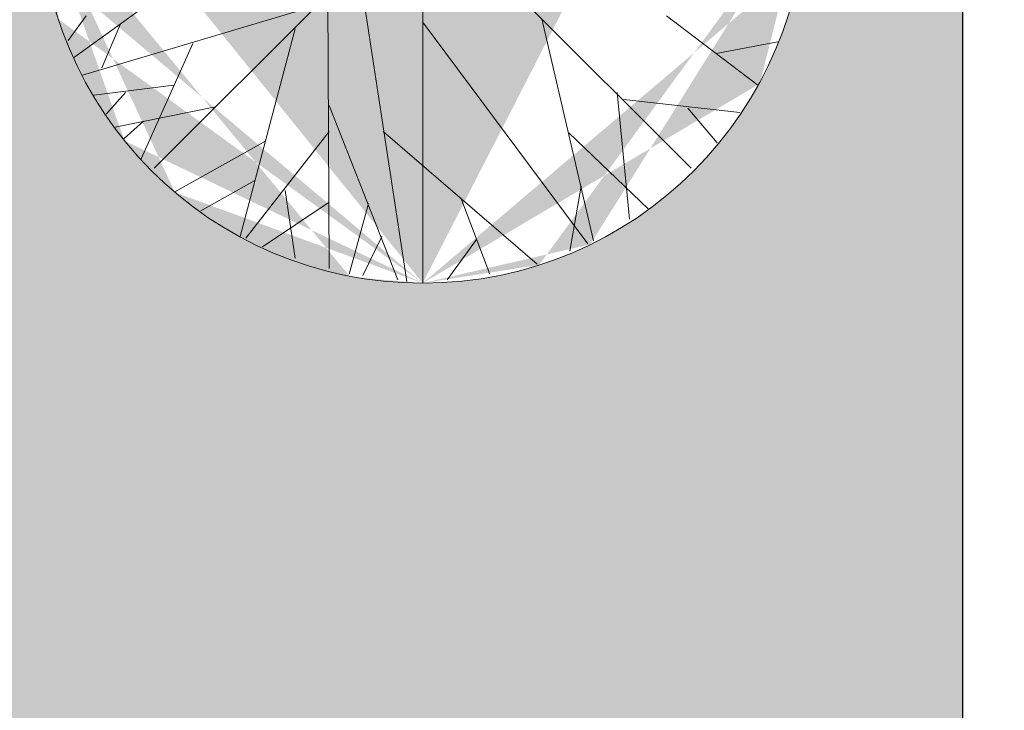
# Model space of a CAD drawing. Units: inches. Extents: x 459864 to 460310, y 324185 to 324787.
# Tile 76 of 112: x 460240 to 460271, y 324238 to 324260. Entities that reach past the tile are written whole.
import ezdxf

# ---------------------------------------------------------------- set-up
doc = ezdxf.new("R2010")
doc.units = ezdxf.units.IN
for name, color, linetype, lineweight in [('A-ANNO-DIMS', 2, 'Continuous', 18), ('C-PROP', 7, 'Continuous', 30), ('L-PLNT', 3, 'Continuous', 13), ('L-SITE-PATT', 252, 'Continuous', 13)]:
    doc.layers.add(name, color=color, linetype=linetype, lineweight=lineweight)
doc.styles.get("Standard").update_dxf_attribs({"font": 'arial.ttf'})
doc.dimstyles.new('ISO-25', dxfattribs={"dimtxt": 6, "dimasz": 2.5, "dimexe": 1.25, "dimexo": 0.625, "dimtad": 1, "dimdec": 1, "dimlunit": 3, "dimtxsty": 'Standard', "dimcen": 2.5, "dimadec": 0, "dimazin": 0, "dimtfac": 1, "dimtdec": 1, "dimtmove": 0, "dimatfit": 3, "dimfxl": 1, "dimarcsym": 0})

# ---------------------------------------------------------------- blocks, each defined once
blk = doc.blocks.new('Tree - deciduous plan')
for p, q in [((0, 59.9996), (0, -60)), ((42, 42), (-42, -42)), ((42, -42), (-42, 42)), ((-54.6162, -24.7335), (-20.2853, 0.0941)), ((-10.074, -10.0627), (-2.5036, -59.7178)), ((-14.8275, -15.0282), (-14.6515, -57.6865)), ((-53.2078, -27.442), (-16.7641, -16.6081)), ((-52.6797, -18.188), (-55.4966, -22.0251)), ((38.1654, -18.188), (52.426, -29.0219)), ((-47.2219, -19.3166), (-50.2148, -26.3135)), ((-0.0388, -19.0909), (25.8415, -53.8495)), ((18.6232, -18.6394), (26.7218, -53.3981)), ((-19.9331, -20.2194), (-28.5599, -52.721)), ((-35.9543, -22.4765), (-44.0529, -40.5329)), ((45.9119, -24.0564), (55.595, -22.2508)), ((-38.9472, -29.0219), (-51.4472, -30.6018)), ((-46.5177, -30.1504), (-49.5106, -33.536)), ((30.419, -30.1504), (32.3556, -50.0125)), ((-14.6515, -32.1818), (-3.912, -59.4922)), ((31.4753, -31.279), (49.6091, -33.3103)), ((-32.4331, -32.4075), (-48.1021, -35.5674)), ((41.5105, -32.6332), (46.088, -38.0501)), ((-43.7008, -34.6645), (-46.6937, -37.373)), ((-14.6515, -36.2445), (-27.6797, -52.9467)), ((-6.2008, -36.2445), (17.919, -57.0094)), ((22.8485, -36.4702), (35.3485, -48.4326)), ((-24.6867, -37.8244), (-38.7712, -45.7241)), ((-26.2712, -43.9185), (-34.7219, -48.6583)), ((-21.5177, -45.4984), (-19.9331, -56.1065)), ((24.7852, -44.8213), (23.0246, -54.978)), ((-14.6515, -47.3041), (-25.0388, -54.3009)), ((-8.4895, -47.5298), (-11.4825, -58.5893)), ((5.9471, -46.6269), (10.5246, -58.5893)), ((-6.3768, -52.721), (-9.3698, -58.815)), ((8.4119, -53.1724), (3.8344, -59.4922))]:
    blk.add_line(p, q)
blk.add_circle((0, 0), 60)
blk = doc.blocks.new('*D65')
at = {"layer": 'A-ANNO-DIMS', "color": 0, "lineweight": -2, "transparency": 16777216}
for p, q in [((460247.74, 324283.483), (460302.765, 324283.483)), ((460301.515, 324280.983), (460301.515, 324197.483)), ((460271.74, 324194.983), (460302.765, 324194.983))]:
    blk.add_line(p, q, dxfattribs=at)
at = {"layer": 'A-ANNO-DIMS', "color": 0, "transparency": 16777216}
for points in [[(460301.098, 324280.983), (460301.932, 324280.983), (460301.515, 324283.483)], [(460301.098, 324197.483), (460301.932, 324197.483), (460301.515, 324194.983)]]:
    blk.add_solid(points, dxfattribs=at)
at = {"layer": 'Defpoints', "color": 0, "transparency": 16777216}
for p in [(460247.115, 324283.483), (460271.115, 324194.983), (460301.515, 324194.983)]:
    blk.add_point(p, dxfattribs=at)
at = {"layer": 'A-ANNO-DIMS', "color": 0, "transparency": 16777216, "insert": (460297.788, 324239.233), "char_height": 6, "attachment_point": 5, "rotation": 90}
blk.add_mtext('7\'-4 1/2"', dxfattribs=at)

msp = doc.modelspace()

# ---------------------------------------------------------------- hatches: boundary and pattern name
at = {"layer": 'L-SITE-PATT'}
h = msp.add_hatch(dxfattribs=at)
h.set_pattern_fill('DOTS', color=256)
h.paths.add_polyline_path([(460269.804, 324283.483), (460247.115, 324283.483), (460121.929, 324283.483), (460121.929, 324252.473), (460117.429, 324252.473), (460110.124, 324252.473), (460110.124, 324243.287), (460080.83, 324243.287), (460080.83, 324252.473), (460061.115, 324252.473), (460061.115, 324251.882), (460077.909, 324251.882), (460077.909, 324199.483), (460080.83, 324199.483), (460080.83, 324207.553), (460110.124, 324207.553), (460110.124, 324199.483), (460110.813, 324199.483), (460262.115, 324199.483), (460269.804, 324199.483)], flags=17)
edge = h.paths.add_edge_path(flags=0)
edge.add_ellipse((460222.59, 324263.813), major_axis=(-8.485, 8.485), ratio=1, start_angle=405, end_angle=495, ccw=False)
edge.add_line((460214.821, 324254.66), (460214.832, 324254.666))
edge.add_ellipse((460222.59, 324263.813), major_axis=(-8.485, 8.485), ratio=1, start_angle=405, end_angle=495, ccw=False)
edge.add_line((460210.759, 324261.781), (460210.768, 324261.787))
edge.add_ellipse((460222.59, 324263.813), major_axis=(-8.485, 8.485), ratio=1, start_angle=405, end_angle=495, ccw=False)
edge.add_ellipse((460222.59, 324263.813), major_axis=(-8.485, 8.485), ratio=1, start_angle=392.754, end_angle=405, ccw=False)
edge.add_ellipse((460222.59, 324263.813), major_axis=(-8.485, 8.485), ratio=1, start_angle=380.9347, end_angle=392.754, ccw=False)
edge.add_line((460211.337, 324267.985), (460211.34, 324267.985))
edge.add_ellipse((460222.59, 324263.813), major_axis=(-8.485, 8.485), ratio=1, start_angle=380.9347, end_angle=392.754, ccw=False)
edge.add_ellipse((460222.59, 324263.813), major_axis=(-8.485, 8.485), ratio=1, start_angle=347.9015, end_angle=380.9347, ccw=False)
edge.add_ellipse((460222.59, 324263.813), major_axis=(-8.485, 8.485), ratio=1, start_angle=327.0619, end_angle=347.9015, ccw=False)
edge.add_ellipse((460222.59, 324263.813), major_axis=(-8.485, 8.485), ratio=1, start_angle=278.3246, end_angle=327.0619, ccw=False)
edge.add_line((460225.158, 324275.536), (460225.158, 324275.535))
edge.add_ellipse((460222.59, 324263.813), major_axis=(-8.485, 8.485), ratio=1, start_angle=278.3246, end_angle=327.0619, ccw=False)
edge.add_ellipse((460222.59, 324263.813), major_axis=(-8.485, 8.485), ratio=1, start_angle=260.6436, end_angle=278.3246, ccw=False)
edge.add_ellipse((460222.59, 324263.813), major_axis=(-8.485, 8.485), ratio=1, start_angle=225, end_angle=260.6436, ccw=False)
edge.add_line((460234.509, 324265.243), (460234.501, 324265.239))
edge.add_ellipse((460222.59, 324263.813), major_axis=(-8.485, 8.485), ratio=1, start_angle=225, end_angle=260.6436, ccw=False)
edge.add_ellipse((460222.59, 324263.813), major_axis=(-8.485, 8.485), ratio=1, start_angle=495, end_angle=585, ccw=False)
edge.add_line((460234.437, 324261.861), (460234.424, 324261.858))
edge.add_ellipse((460222.59, 324263.813), major_axis=(-8.485, 8.485), ratio=1, start_angle=495, end_angle=585, ccw=False)
edge.add_line((460227.95, 324253.067), (460227.946, 324253.083))
edge.add_ellipse((460222.59, 324263.813), major_axis=(-8.485, 8.485), ratio=1, start_angle=495, end_angle=585, ccw=False)
edge.add_line((460226.223, 324252.369), (460226.211, 324252.38))
edge.add_ellipse((460222.59, 324263.813), major_axis=(-8.485, 8.485), ratio=1, start_angle=495, end_angle=585, ccw=False)
h.paths.add_polyline_path([(460219.651, 324254.347), (460218.461, 324253.545), (460218.275, 324254.789), (460219.642, 324256.542), (460219.625, 324260.848), (460216.11, 324257.333), (460214.35, 324256.978), (460215.416, 324259.356), (460212.524, 324258.496), (460213.137, 324259.93), (460218.507, 324263.813), (460222.59, 324263.813), (460222.59, 324267.807), (460218.176, 324272.212), (460219.026, 324274.639), (460222.59, 324272.811), (460222.59, 324275.423), (460223.057, 324274.825), (460222.675, 324273.492), (460225.912, 324267.135), (460219.625, 324260.848)], flags=0)
edge = h.paths.add_edge_path(flags=0)
edge.add_ellipse((460194.576, 324264.046), major_axis=(-8.485, 8.485), ratio=1, start_angle=495, end_angle=585, ccw=False)
edge.add_line((460199.936, 324253.3), (460199.932, 324253.316))
edge.add_ellipse((460194.576, 324264.046), major_axis=(-8.485, 8.485), ratio=1, start_angle=495, end_angle=585, ccw=False)
edge.add_line((460198.208, 324252.603), (460198.196, 324252.613))
edge.add_ellipse((460194.576, 324264.046), major_axis=(-8.485, 8.485), ratio=1, start_angle=495, end_angle=585, ccw=False)
edge.add_ellipse((460194.576, 324264.046), major_axis=(-8.485, 8.485), ratio=1, start_angle=405, end_angle=495, ccw=False)
edge.add_line((460186.806, 324254.893), (460186.817, 324254.899))
edge.add_ellipse((460194.576, 324264.046), major_axis=(-8.485, 8.485), ratio=1, start_angle=405, end_angle=495, ccw=False)
edge.add_line((460182.744, 324262.014), (460182.753, 324262.02))
edge.add_ellipse((460194.576, 324264.046), major_axis=(-8.485, 8.485), ratio=1, start_angle=405, end_angle=495, ccw=False)
edge.add_ellipse((460194.576, 324264.046), major_axis=(-8.485, 8.485), ratio=1, start_angle=392.754, end_angle=405, ccw=False)
edge.add_ellipse((460194.576, 324264.046), major_axis=(-8.485, 8.485), ratio=1, start_angle=380.9347, end_angle=392.754, ccw=False)
edge.add_line((460183.323, 324268.218), (460183.326, 324268.218))
edge.add_ellipse((460194.576, 324264.046), major_axis=(-8.485, 8.485), ratio=1, start_angle=380.9347, end_angle=392.754, ccw=False)
edge.add_ellipse((460194.576, 324264.046), major_axis=(-8.485, 8.485), ratio=1, start_angle=347.9015, end_angle=380.9347, ccw=False)
edge.add_ellipse((460194.576, 324264.046), major_axis=(-8.485, 8.485), ratio=1, start_angle=327.0619, end_angle=347.9015, ccw=False)
edge.add_ellipse((460194.576, 324264.046), major_axis=(-8.485, 8.485), ratio=1, start_angle=278.3246, end_angle=327.0619, ccw=False)
edge.add_line((460197.144, 324275.769), (460197.143, 324275.768))
edge.add_ellipse((460194.576, 324264.046), major_axis=(-8.485, 8.485), ratio=1, start_angle=278.3246, end_angle=327.0619, ccw=False)
edge.add_ellipse((460194.576, 324264.046), major_axis=(-8.485, 8.485), ratio=1, start_angle=260.6436, end_angle=278.3246, ccw=False)
edge.add_ellipse((460194.576, 324264.046), major_axis=(-8.485, 8.485), ratio=1, start_angle=225, end_angle=260.6436, ccw=False)
edge.add_line((460206.494, 324265.476), (460206.487, 324265.473))
edge.add_ellipse((460194.576, 324264.046), major_axis=(-8.485, 8.485), ratio=1, start_angle=225, end_angle=260.6436, ccw=False)
edge.add_ellipse((460194.576, 324264.046), major_axis=(-8.485, 8.485), ratio=1, start_angle=495, end_angle=585, ccw=False)
edge.add_line((460206.422, 324262.094), (460206.409, 324262.091))
h.paths.add_polyline_path([(460191.61, 324261.081), (460191.637, 324254.58), (460190.447, 324253.778), (460190.261, 324255.023), (460191.628, 324256.775), (460191.61, 324261.081), (460188.096, 324257.566), (460186.335, 324257.211), (460187.402, 324259.589), (460184.509, 324258.729), (460185.123, 324260.163), (460190.493, 324264.046), (460194.576, 324264.046), (460194.576, 324268.04), (460190.161, 324272.446), (460191.011, 324274.872), (460194.576, 324273.044), (460194.576, 324275.657), (460195.043, 324275.058), (460194.661, 324273.725), (460197.897, 324267.368)], flags=0)
edge = h.paths.add_edge_path(flags=0)
edge.add_ellipse((460252.912, 324263.578), major_axis=(-8.485, 8.485), ratio=1, start_angle=405, end_angle=495, ccw=False)
edge.add_line((460241.081, 324261.545), (460241.089, 324261.551))
edge.add_ellipse((460252.912, 324263.578), major_axis=(-8.485, 8.485), ratio=1, start_angle=405, end_angle=495, ccw=False)
edge.add_ellipse((460252.912, 324263.578), major_axis=(-8.485, 8.485), ratio=1, start_angle=392.754, end_angle=405, ccw=False)
edge.add_ellipse((460252.912, 324263.578), major_axis=(-8.485, 8.485), ratio=1, start_angle=380.9347, end_angle=392.754, ccw=False)
edge.add_line((460241.659, 324267.749), (460241.662, 324267.749))
edge.add_ellipse((460252.912, 324263.578), major_axis=(-8.485, 8.485), ratio=1, start_angle=380.9347, end_angle=392.754, ccw=False)
edge.add_ellipse((460252.912, 324263.578), major_axis=(-8.485, 8.485), ratio=1, start_angle=347.9015, end_angle=380.9347, ccw=False)
edge.add_ellipse((460252.912, 324263.578), major_axis=(-8.485, 8.485), ratio=1, start_angle=327.0619, end_angle=347.9015, ccw=False)
edge.add_ellipse((460252.912, 324263.578), major_axis=(-8.485, 8.485), ratio=1, start_angle=278.3246, end_angle=327.0619, ccw=False)
edge.add_line((460255.48, 324275.3), (460255.479, 324275.299))
edge.add_ellipse((460252.912, 324263.578), major_axis=(-8.485, 8.485), ratio=1, start_angle=278.3246, end_angle=327.0619, ccw=False)
edge.add_ellipse((460252.912, 324263.578), major_axis=(-8.485, 8.485), ratio=1, start_angle=260.6436, end_angle=278.3246, ccw=False)
edge.add_ellipse((460252.912, 324263.578), major_axis=(-8.485, 8.485), ratio=1, start_angle=225, end_angle=260.6436, ccw=False)
edge.add_line((460264.83, 324265.007), (460264.823, 324265.004))
edge.add_ellipse((460252.912, 324263.578), major_axis=(-8.485, 8.485), ratio=1, start_angle=225, end_angle=260.6436, ccw=False)
edge.add_ellipse((460252.912, 324263.578), major_axis=(-8.485, 8.485), ratio=1, start_angle=495, end_angle=585, ccw=False)
edge.add_line((460264.758, 324261.626), (460264.745, 324261.622))
edge.add_ellipse((460252.912, 324263.578), major_axis=(-8.485, 8.485), ratio=1, start_angle=495, end_angle=585, ccw=False)
edge.add_line((460258.272, 324252.832), (460258.268, 324252.848))
edge.add_ellipse((460252.912, 324263.578), major_axis=(-8.485, 8.485), ratio=1, start_angle=495, end_angle=585, ccw=False)
edge.add_line((460256.545, 324252.134), (460256.533, 324252.144))
edge.add_ellipse((460252.912, 324263.578), major_axis=(-8.485, 8.485), ratio=1, start_angle=495, end_angle=585, ccw=False)
edge.add_ellipse((460252.912, 324263.578), major_axis=(-8.485, 8.485), ratio=1, start_angle=405, end_angle=495, ccw=False)
edge.add_line((460245.143, 324254.424), (460245.153, 324254.43))
h.paths.add_polyline_path([(460244.672, 324256.742), (460245.738, 324259.12), (460242.846, 324258.26), (460243.459, 324259.694), (460248.829, 324263.578), (460252.912, 324263.578), (460252.912, 324267.571), (460248.497, 324271.977), (460249.348, 324274.403), (460252.912, 324272.576), (460252.912, 324275.188), (460253.379, 324274.589), (460252.997, 324273.257), (460256.233, 324266.899), (460249.946, 324260.612), (460249.973, 324254.111), (460248.783, 324253.309), (460248.597, 324254.554), (460249.964, 324256.306), (460249.946, 324260.612), (460246.432, 324257.097)], flags=0)
edge = h.paths.add_edge_path(flags=0)
edge.add_ellipse((460167.439, 324262.833), major_axis=(-8.485, 8.485), ratio=1, start_angle=495, end_angle=585, ccw=False)
edge.add_line((460172.799, 324252.087), (460172.795, 324252.103))
edge.add_ellipse((460167.439, 324262.833), major_axis=(-8.485, 8.485), ratio=1, start_angle=495, end_angle=585, ccw=False)
edge.add_line((460171.071, 324251.389), (460171.059, 324251.399))
edge.add_ellipse((460167.439, 324262.833), major_axis=(-8.485, 8.485), ratio=1, start_angle=495, end_angle=585, ccw=False)
edge.add_ellipse((460167.439, 324262.833), major_axis=(-8.485, 8.485), ratio=1, start_angle=405, end_angle=495, ccw=False)
edge.add_line((460159.669, 324253.679), (460159.68, 324253.685))
edge.add_ellipse((460167.439, 324262.833), major_axis=(-8.485, 8.485), ratio=1, start_angle=405, end_angle=495, ccw=False)
edge.add_line((460155.607, 324260.8), (460155.616, 324260.806))
edge.add_ellipse((460167.439, 324262.833), major_axis=(-8.485, 8.485), ratio=1, start_angle=405, end_angle=495, ccw=False)
edge.add_ellipse((460167.439, 324262.833), major_axis=(-8.485, 8.485), ratio=1, start_angle=392.754, end_angle=405, ccw=False)
edge.add_ellipse((460167.439, 324262.833), major_axis=(-8.485, 8.485), ratio=1, start_angle=380.9347, end_angle=392.754, ccw=False)
edge.add_line((460156.185, 324267.005), (460156.189, 324267.005))
edge.add_ellipse((460167.439, 324262.833), major_axis=(-8.485, 8.485), ratio=1, start_angle=380.9347, end_angle=392.754, ccw=False)
edge.add_ellipse((460167.439, 324262.833), major_axis=(-8.485, 8.485), ratio=1, start_angle=347.9015, end_angle=380.9347, ccw=False)
edge.add_ellipse((460167.439, 324262.833), major_axis=(-8.485, 8.485), ratio=1, start_angle=327.0619, end_angle=347.9015, ccw=False)
edge.add_ellipse((460167.439, 324262.833), major_axis=(-8.485, 8.485), ratio=1, start_angle=278.3246, end_angle=327.0619, ccw=False)
edge.add_line((460170.007, 324274.556), (460170.006, 324274.554))
edge.add_ellipse((460167.439, 324262.833), major_axis=(-8.485, 8.485), ratio=1, start_angle=278.3246, end_angle=327.0619, ccw=False)
edge.add_ellipse((460167.439, 324262.833), major_axis=(-8.485, 8.485), ratio=1, start_angle=260.6436, end_angle=278.3246, ccw=False)
edge.add_ellipse((460167.439, 324262.833), major_axis=(-8.485, 8.485), ratio=1, start_angle=225, end_angle=260.6436, ccw=False)
edge.add_line((460179.357, 324264.262), (460179.35, 324264.259))
edge.add_ellipse((460167.439, 324262.833), major_axis=(-8.485, 8.485), ratio=1, start_angle=225, end_angle=260.6436, ccw=False)
edge.add_ellipse((460167.439, 324262.833), major_axis=(-8.485, 8.485), ratio=1, start_angle=495, end_angle=585, ccw=False)
edge.add_line((460179.285, 324260.881), (460179.272, 324260.877))
h.paths.add_polyline_path([(460164.473, 324259.867), (460164.5, 324253.366), (460163.31, 324252.565), (460163.124, 324253.809), (460164.491, 324255.561), (460164.473, 324259.867), (460160.958, 324256.353), (460159.198, 324255.998), (460160.265, 324258.375), (460157.372, 324257.515), (460157.986, 324258.949), (460163.356, 324262.833), (460167.439, 324262.833), (460167.439, 324266.826), (460163.024, 324271.232), (460163.874, 324273.659), (460167.439, 324271.831), (460167.439, 324274.443), (460167.905, 324273.844), (460167.524, 324272.512), (460170.76, 324266.154)], flags=0)
edge = h.paths.add_edge_path(flags=0)
edge.add_ellipse((460140.758, 324262.37), major_axis=(-8.485, 8.485), ratio=1, start_angle=495, end_angle=585, ccw=False)
edge.add_line((460146.118, 324251.624), (460146.114, 324251.639))
edge.add_ellipse((460140.758, 324262.37), major_axis=(-8.485, 8.485), ratio=1, start_angle=495, end_angle=585, ccw=False)
edge.add_line((460144.391, 324250.926), (460144.379, 324250.936))
edge.add_ellipse((460140.758, 324262.37), major_axis=(-8.485, 8.485), ratio=1, start_angle=495, end_angle=585, ccw=False)
edge.add_ellipse((460140.758, 324262.37), major_axis=(-8.485, 8.485), ratio=1, start_angle=405, end_angle=495, ccw=False)
edge.add_line((460132.989, 324253.216), (460132.999, 324253.222))
edge.add_ellipse((460140.758, 324262.37), major_axis=(-8.485, 8.485), ratio=1, start_angle=405, end_angle=495, ccw=False)
edge.add_line((460128.927, 324260.337), (460128.935, 324260.343))
edge.add_ellipse((460140.758, 324262.37), major_axis=(-8.485, 8.485), ratio=1, start_angle=405, end_angle=495, ccw=False)
edge.add_ellipse((460140.758, 324262.37), major_axis=(-8.485, 8.485), ratio=1, start_angle=392.754, end_angle=405, ccw=False)
edge.add_ellipse((460140.758, 324262.37), major_axis=(-8.485, 8.485), ratio=1, start_angle=380.9347, end_angle=392.754, ccw=False)
edge.add_line((460129.505, 324266.541), (460129.508, 324266.541))
edge.add_ellipse((460140.758, 324262.37), major_axis=(-8.485, 8.485), ratio=1, start_angle=380.9347, end_angle=392.754, ccw=False)
edge.add_ellipse((460140.758, 324262.37), major_axis=(-8.485, 8.485), ratio=1, start_angle=347.9015, end_angle=380.9347, ccw=False)
edge.add_ellipse((460140.758, 324262.37), major_axis=(-8.485, 8.485), ratio=1, start_angle=327.0619, end_angle=347.9015, ccw=False)
edge.add_ellipse((460140.758, 324262.37), major_axis=(-8.485, 8.485), ratio=1, start_angle=278.3246, end_angle=327.0619, ccw=False)
edge.add_line((460143.326, 324274.092), (460143.325, 324274.091))
edge.add_ellipse((460140.758, 324262.37), major_axis=(-8.485, 8.485), ratio=1, start_angle=278.3246, end_angle=327.0619, ccw=False)
edge.add_ellipse((460140.758, 324262.37), major_axis=(-8.485, 8.485), ratio=1, start_angle=260.6436, end_angle=278.3246, ccw=False)
edge.add_ellipse((460140.758, 324262.37), major_axis=(-8.485, 8.485), ratio=1, start_angle=225, end_angle=260.6436, ccw=False)
edge.add_line((460152.677, 324263.799), (460152.669, 324263.796))
edge.add_ellipse((460140.758, 324262.37), major_axis=(-8.485, 8.485), ratio=1, start_angle=225, end_angle=260.6436, ccw=False)
edge.add_ellipse((460140.758, 324262.37), major_axis=(-8.485, 8.485), ratio=1, start_angle=495, end_angle=585, ccw=False)
edge.add_line((460152.604, 324260.418), (460152.592, 324260.414))
h.paths.add_polyline_path([(460137.792, 324259.404), (460137.819, 324252.903), (460136.629, 324252.101), (460136.443, 324253.346), (460137.81, 324255.098), (460137.792, 324259.404), (460134.278, 324255.889), (460132.518, 324255.534), (460133.584, 324257.912), (460130.692, 324257.052), (460131.305, 324258.486), (460136.675, 324262.37), (460140.758, 324262.37), (460140.758, 324266.363), (460136.343, 324270.769), (460137.194, 324273.195), (460140.758, 324271.367), (460140.758, 324273.98), (460141.225, 324273.381), (460140.843, 324272.049), (460144.079, 324265.691)], flags=0)
h.paths.add_polyline_path([(460110.124, 324227.414), (460080.83, 324227.414), (460080.83, 324235.484), (460110.124, 324235.484)], flags=16)
h.paths.add_polyline_path([(460110.124, 324220.797), (460110.124, 324212.727), (460080.83, 324212.727), (460080.83, 324220.797)], flags=16)
h.paths.add_polyline_path([(460269.804, 324283.483), (460247.115, 324283.483), (460121.929, 324283.483), (460121.929, 324252.473), (460117.429, 324252.473), (460110.124, 324252.473), (460110.124, 324243.287), (460080.83, 324243.287), (460080.83, 324252.473), (460061.115, 324252.473), (460061.115, 324251.882), (460077.909, 324251.882), (460077.909, 324199.483), (460080.83, 324199.483), (460080.83, 324207.553), (460110.124, 324207.553), (460110.124, 324199.483), (460262.115, 324199.483), (460269.804, 324199.483)], flags=17)
h.paths.add_polyline_path([(460219.651, 324254.347), (460218.461, 324253.545), (460218.275, 324254.789), (460219.642, 324256.542), (460219.625, 324260.848), (460216.11, 324257.333), (460214.35, 324256.978), (460215.416, 324259.356), (460212.524, 324258.496), (460213.137, 324259.93), (460218.507, 324263.813), (460222.59, 324263.813), (460220.18, 324266.223), (460215.461, 324265.308), (460211.835, 324266.137), (460216.247, 324267.985), (460218.418, 324267.985), (460222.59, 324263.813), (460222.59, 324267.807), (460218.176, 324272.212), (460219.026, 324274.639), (460222.59, 324272.811), (460222.59, 324275.423), (460223.057, 324274.825), (460222.675, 324273.492), (460225.912, 324267.135), (460222.59, 324263.813), (460231.383, 324263.813), (460228.485, 324262.488), (460224.425, 324261.978), (460228.68, 324257.724), (460228.966, 324254.791), (460227.142, 324256.537), (460227.542, 324254.819), (460227.333, 324253.614), (460222.59, 324259.985), (460222.59, 324255.497), (460221.377, 324256.541), (460220.576, 324261.799), (460219.625, 324260.848)], flags=0)
h.paths.add_polyline_path([(460199.127, 324256.77), (460199.528, 324255.052), (460199.319, 324253.848), (460194.576, 324260.218), (460194.576, 324255.73), (460193.363, 324256.774), (460192.561, 324262.032), (460191.61, 324261.081), (460191.637, 324254.58), (460190.447, 324253.778), (460190.261, 324255.023), (460191.628, 324256.775), (460191.61, 324261.081), (460188.096, 324257.566), (460186.335, 324257.211), (460187.402, 324259.589), (460184.509, 324258.729), (460185.123, 324260.163), (460190.493, 324264.046), (460194.576, 324264.046), (460192.166, 324266.456), (460187.446, 324265.541), (460183.82, 324266.37), (460188.232, 324268.218), (460190.404, 324268.218), (460194.576, 324264.046), (460194.576, 324268.04), (460190.161, 324272.446), (460191.011, 324274.872), (460194.576, 324273.044), (460194.576, 324275.657), (460195.043, 324275.058), (460194.661, 324273.725), (460197.897, 324267.368), (460194.576, 324264.046), (460203.368, 324264.046), (460200.47, 324262.721), (460196.411, 324262.212), (460200.665, 324257.957), (460200.951, 324255.024)], flags=0)
h.paths.add_polyline_path([(460244.672, 324256.742), (460245.738, 324259.12), (460242.846, 324258.26), (460243.459, 324259.694), (460248.829, 324263.578), (460252.912, 324263.578), (460250.502, 324265.987), (460245.783, 324265.072), (460242.156, 324265.901), (460246.568, 324267.749), (460248.74, 324267.749), (460252.912, 324263.578), (460252.912, 324267.571), (460248.497, 324271.977), (460249.348, 324274.403), (460252.912, 324272.576), (460252.912, 324275.188), (460253.379, 324274.589), (460252.997, 324273.257), (460256.233, 324266.899), (460252.912, 324263.578), (460261.705, 324263.578), (460258.806, 324262.252), (460254.747, 324261.743), (460259.002, 324257.488), (460259.288, 324254.555), (460257.463, 324256.301), (460257.864, 324254.583), (460257.655, 324253.379), (460252.912, 324259.749), (460252.912, 324255.261), (460251.699, 324256.305), (460250.897, 324261.563), (460249.946, 324260.612), (460249.973, 324254.111), (460248.783, 324253.309), (460248.597, 324254.554), (460249.964, 324256.306), (460249.946, 324260.612), (460246.432, 324257.097)], flags=0)
h.paths.add_polyline_path([(460173.528, 324256.743), (460173.814, 324253.811), (460171.99, 324255.556), (460172.39, 324253.838), (460172.182, 324252.634), (460167.439, 324259.004), (460167.439, 324254.516), (460166.226, 324255.56), (460165.424, 324260.818), (460164.473, 324259.867), (460164.5, 324253.366), (460163.31, 324252.565), (460163.124, 324253.809), (460164.491, 324255.561), (460164.473, 324259.867), (460160.958, 324256.353), (460159.198, 324255.998), (460160.265, 324258.375), (460157.372, 324257.515), (460157.986, 324258.949), (460163.356, 324262.833), (460167.439, 324262.833), (460165.029, 324265.243), (460160.309, 324264.327), (460156.683, 324265.156), (460161.095, 324267.005), (460163.267, 324267.005), (460167.439, 324262.833), (460167.439, 324266.826), (460163.024, 324271.232), (460163.874, 324273.659), (460167.439, 324271.831), (460167.439, 324274.443), (460167.905, 324273.844), (460167.524, 324272.512), (460170.76, 324266.154), (460167.439, 324262.833), (460176.231, 324262.833), (460173.333, 324261.507), (460169.274, 324260.998)], flags=0)
h.paths.add_polyline_path([(460146.848, 324256.28), (460147.134, 324253.347), (460145.31, 324255.093), (460145.71, 324253.375), (460145.501, 324252.171), (460140.758, 324258.541), (460140.758, 324254.053), (460139.545, 324255.097), (460138.744, 324260.355), (460137.792, 324259.404), (460137.819, 324252.903), (460136.629, 324252.101), (460136.443, 324253.346), (460137.81, 324255.098), (460137.792, 324259.404), (460134.278, 324255.889), (460132.518, 324255.534), (460133.584, 324257.912), (460130.692, 324257.052), (460131.305, 324258.486), (460136.675, 324262.37), (460140.758, 324262.37), (460138.348, 324264.779), (460133.629, 324263.864), (460130.002, 324264.693), (460134.414, 324266.541), (460136.586, 324266.541), (460140.758, 324262.37), (460140.758, 324266.363), (460136.343, 324270.769), (460137.194, 324273.195), (460140.758, 324271.367), (460140.758, 324273.98), (460141.225, 324273.381), (460140.843, 324272.049), (460144.079, 324265.691), (460140.758, 324262.37), (460149.551, 324262.37), (460146.653, 324261.044), (460142.593, 324260.535)], flags=0)
edge = h.paths.add_edge_path()
edge.add_line((460269.804, 324272.549), (460260.881, 324272.549))
edge.add_ellipse((460252.912, 324263.578), major_axis=(-8.485, 8.485), ratio=1, start_angle=260.6436, end_angle=273.3846, ccw=False)
edge.add_line((460262.283, 324271.092), (460262.261, 324271.091))
edge.add_ellipse((460252.912, 324263.578), major_axis=(-8.485, 8.485), ratio=1, start_angle=260.6436, end_angle=273.3846, ccw=False)
edge.add_ellipse((460252.912, 324263.578), major_axis=(-8.485, 8.485), ratio=1, start_angle=225, end_angle=260.6436, ccw=False)
edge.add_line((460263.609, 324269.063), (460263.572, 324269.058))
edge.add_ellipse((460252.912, 324263.578), major_axis=(-8.485, 8.485), ratio=1, start_angle=225, end_angle=260.6436, ccw=False)
edge.add_line((460264.615, 324266.306), (460264.585, 324266.305))
edge.add_ellipse((460252.912, 324263.578), major_axis=(-8.485, 8.485), ratio=1, start_angle=225, end_angle=260.6436, ccw=False)
edge.add_line((460264.83, 324265.007), (460264.823, 324265.004))
edge.add_ellipse((460252.912, 324263.578), major_axis=(-8.485, 8.485), ratio=1, start_angle=225, end_angle=260.6436, ccw=False)
edge.add_ellipse((460252.912, 324263.578), major_axis=(-8.485, 8.485), ratio=1, start_angle=495, end_angle=585, ccw=False)
edge.add_line((460264.758, 324261.626), (460264.745, 324261.622))
edge.add_ellipse((460252.912, 324263.578), major_axis=(-8.485, 8.485), ratio=1, start_angle=495, end_angle=585, ccw=False)
edge.add_line((460263.442, 324257.739), (460263.389, 324257.779))
edge.add_ellipse((460252.912, 324263.578), major_axis=(-8.485, 8.485), ratio=1, start_angle=495, end_angle=585, ccw=False)
edge.add_line((460258.128, 324252.744), (460258.102, 324252.779))
edge.add_ellipse((460252.912, 324263.578), major_axis=(-8.485, 8.485), ratio=1, start_angle=495, end_angle=585, ccw=False)
edge.add_line((460256.545, 324252.134), (460256.533, 324252.144))
edge.add_ellipse((460252.912, 324263.578), major_axis=(-8.485, 8.485), ratio=1, start_angle=495, end_angle=585, ccw=False)
edge.add_ellipse((460252.912, 324263.578), major_axis=(-8.485, 8.485), ratio=1, start_angle=405, end_angle=495, ccw=False)
edge.add_line((460250.594, 324251.78), (460250.605, 324251.82))
edge.add_ellipse((460252.912, 324263.578), major_axis=(-8.485, 8.485), ratio=1, start_angle=405, end_angle=495, ccw=False)
edge.add_line((460245.143, 324254.424), (460245.153, 324254.43))
edge.add_ellipse((460252.912, 324263.578), major_axis=(-8.485, 8.485), ratio=1, start_angle=405, end_angle=495, ccw=False)
edge.add_line((460243.525, 324256.059), (460243.56, 324256.091))
edge.add_ellipse((460252.912, 324263.578), major_axis=(-8.485, 8.485), ratio=1, start_angle=405, end_angle=495, ccw=False)
edge.add_line((460241.44, 324259.893), (460241.522, 324259.896))
edge.add_ellipse((460252.912, 324263.578), major_axis=(-8.485, 8.485), ratio=1, start_angle=405, end_angle=495, ccw=False)
edge.add_line((460241.081, 324261.545), (460241.089, 324261.551))
edge.add_ellipse((460252.912, 324263.578), major_axis=(-8.485, 8.485), ratio=1, start_angle=405, end_angle=495, ccw=False)
edge.add_ellipse((460252.912, 324263.578), major_axis=(-8.485, 8.485), ratio=1, start_angle=392.754, end_angle=405, ccw=False)
edge.add_line((460241.05, 324265.438), (460241.063, 324265.443))
edge.add_ellipse((460252.912, 324263.578), major_axis=(-8.485, 8.485), ratio=1, start_angle=392.754, end_angle=405, ccw=False)
edge.add_ellipse((460252.912, 324263.578), major_axis=(-8.485, 8.485), ratio=1, start_angle=380.9347, end_angle=392.754, ccw=False)
edge.add_line((460241.452, 324267.176), (460241.469, 324267.171))
edge.add_ellipse((460252.912, 324263.578), major_axis=(-8.485, 8.485), ratio=1, start_angle=380.9347, end_angle=392.754, ccw=False)
edge.add_line((460241.659, 324267.749), (460241.662, 324267.749))
edge.add_ellipse((460252.912, 324263.578), major_axis=(-8.485, 8.485), ratio=1, start_angle=380.9347, end_angle=392.754, ccw=False)
edge.add_ellipse((460252.912, 324263.578), major_axis=(-8.485, 8.485), ratio=1, start_angle=356.6154, end_angle=380.9347, ccw=False)
edge.add_line((460244.88, 324272.488), (460244.713, 324272.549))
edge.add_line((460244.713, 324272.549), (460230.817, 324272.549))
edge.add_ellipse((460222.59, 324263.813), major_axis=(-8.485, 8.485), ratio=1, start_angle=260.6436, end_angle=271.7178, ccw=False)
edge.add_ellipse((460222.59, 324263.813), major_axis=(-8.485, 8.485), ratio=1, start_angle=225, end_angle=260.6436, ccw=False)
edge.add_line((460233.287, 324269.299), (460233.25, 324269.294))
edge.add_ellipse((460222.59, 324263.813), major_axis=(-8.485, 8.485), ratio=1, start_angle=225, end_angle=260.6436, ccw=False)
edge.add_line((460234.294, 324266.541), (460234.264, 324266.541))
edge.add_ellipse((460222.59, 324263.813), major_axis=(-8.485, 8.485), ratio=1, start_angle=225, end_angle=260.6436, ccw=False)
edge.add_line((460234.509, 324265.243), (460234.501, 324265.239))
edge.add_ellipse((460222.59, 324263.813), major_axis=(-8.485, 8.485), ratio=1, start_angle=225, end_angle=260.6436, ccw=False)
edge.add_ellipse((460222.59, 324263.813), major_axis=(-8.485, 8.485), ratio=1, start_angle=495, end_angle=585, ccw=False)
edge.add_line((460234.437, 324261.861), (460234.424, 324261.858))
edge.add_ellipse((460222.59, 324263.813), major_axis=(-8.485, 8.485), ratio=1, start_angle=495, end_angle=585, ccw=False)
edge.add_line((460233.121, 324257.975), (460233.068, 324258.015))
edge.add_ellipse((460222.59, 324263.813), major_axis=(-8.485, 8.485), ratio=1, start_angle=495, end_angle=585, ccw=False)
edge.add_line((460227.806, 324252.979), (460227.78, 324253.014))
edge.add_ellipse((460222.59, 324263.813), major_axis=(-8.485, 8.485), ratio=1, start_angle=495, end_angle=585, ccw=False)
edge.add_line((460226.223, 324252.369), (460226.211, 324252.38))
edge.add_ellipse((460222.59, 324263.813), major_axis=(-8.485, 8.485), ratio=1, start_angle=495, end_angle=585, ccw=False)
edge.add_ellipse((460222.59, 324263.813), major_axis=(-8.485, 8.485), ratio=1, start_angle=405, end_angle=495, ccw=False)
edge.add_line((460220.272, 324252.016), (460220.283, 324252.055))
edge.add_ellipse((460222.59, 324263.813), major_axis=(-8.485, 8.485), ratio=1, start_angle=405, end_angle=495, ccw=False)
edge.add_line((460214.821, 324254.66), (460214.832, 324254.666))
edge.add_ellipse((460222.59, 324263.813), major_axis=(-8.485, 8.485), ratio=1, start_angle=405, end_angle=495, ccw=False)
edge.add_line((460213.203, 324256.295), (460213.239, 324256.327))
edge.add_ellipse((460222.59, 324263.813), major_axis=(-8.485, 8.485), ratio=1, start_angle=405, end_angle=495, ccw=False)
edge.add_line((460211.118, 324260.128), (460211.201, 324260.131))
edge.add_ellipse((460222.59, 324263.813), major_axis=(-8.485, 8.485), ratio=1, start_angle=405, end_angle=495, ccw=False)
edge.add_line((460210.759, 324261.781), (460210.768, 324261.787))
edge.add_ellipse((460222.59, 324263.813), major_axis=(-8.485, 8.485), ratio=1, start_angle=405, end_angle=495, ccw=False)
edge.add_ellipse((460222.59, 324263.813), major_axis=(-8.485, 8.485), ratio=1, start_angle=392.754, end_angle=405, ccw=False)
edge.add_line((460210.729, 324265.673), (460210.741, 324265.678))
edge.add_ellipse((460222.59, 324263.813), major_axis=(-8.485, 8.485), ratio=1, start_angle=392.754, end_angle=405, ccw=False)
edge.add_ellipse((460222.59, 324263.813), major_axis=(-8.485, 8.485), ratio=1, start_angle=380.9347, end_angle=392.754, ccw=False)
edge.add_line((460211.13, 324267.412), (460211.147, 324267.407))
edge.add_ellipse((460222.59, 324263.813), major_axis=(-8.485, 8.485), ratio=1, start_angle=380.9347, end_angle=392.754, ccw=False)
edge.add_line((460211.337, 324267.985), (460211.34, 324267.985))
edge.add_ellipse((460222.59, 324263.813), major_axis=(-8.485, 8.485), ratio=1, start_angle=380.9347, end_angle=392.754, ccw=False)
edge.add_ellipse((460222.59, 324263.813), major_axis=(-8.485, 8.485), ratio=1, start_angle=358.2822, end_angle=380.9347, ccw=False)
edge.add_line((460213.705, 324271.902), (460213.709, 324271.869))
edge.add_ellipse((460222.59, 324263.813), major_axis=(-8.485, 8.485), ratio=1, start_angle=358.2822, end_angle=380.9347, ccw=False)
edge.add_line((460214.363, 324272.549), (460203.078, 324272.549))
edge.add_line((460203.078, 324272.549), (460203.06, 324272.531))
edge.add_ellipse((460194.576, 324264.046), major_axis=(-8.485, 8.485), ratio=1, start_angle=260.6436, end_angle=270.1168, ccw=False)
edge.add_line((460203.957, 324271.561), (460203.921, 324271.56))
edge.add_ellipse((460194.576, 324264.046), major_axis=(-8.485, 8.485), ratio=1, start_angle=260.6436, end_angle=270.1168, ccw=False)
edge.add_ellipse((460194.576, 324264.046), major_axis=(-8.485, 8.485), ratio=1, start_angle=225, end_angle=260.6436, ccw=False)
edge.add_line((460205.272, 324269.532), (460205.235, 324269.527))
edge.add_ellipse((460194.576, 324264.046), major_axis=(-8.485, 8.485), ratio=1, start_angle=225, end_angle=260.6436, ccw=False)
edge.add_line((460206.279, 324266.774), (460206.249, 324266.774))
edge.add_ellipse((460194.576, 324264.046), major_axis=(-8.485, 8.485), ratio=1, start_angle=225, end_angle=260.6436, ccw=False)
edge.add_line((460206.494, 324265.476), (460206.487, 324265.473))
edge.add_ellipse((460194.576, 324264.046), major_axis=(-8.485, 8.485), ratio=1, start_angle=225, end_angle=260.6436, ccw=False)
edge.add_ellipse((460194.576, 324264.046), major_axis=(-8.485, 8.485), ratio=1, start_angle=495, end_angle=585, ccw=False)
edge.add_line((460206.422, 324262.094), (460206.409, 324262.091))
edge.add_ellipse((460194.576, 324264.046), major_axis=(-8.485, 8.485), ratio=1, start_angle=495, end_angle=585, ccw=False)
edge.add_line((460205.106, 324258.208), (460205.053, 324258.248))
edge.add_ellipse((460194.576, 324264.046), major_axis=(-8.485, 8.485), ratio=1, start_angle=495, end_angle=585, ccw=False)
edge.add_line((460199.792, 324253.212), (460199.766, 324253.248))
edge.add_ellipse((460194.576, 324264.046), major_axis=(-8.485, 8.485), ratio=1, start_angle=495, end_angle=585, ccw=False)
edge.add_line((460198.208, 324252.603), (460198.196, 324252.613))
edge.add_ellipse((460194.576, 324264.046), major_axis=(-8.485, 8.485), ratio=1, start_angle=495, end_angle=585, ccw=False)
edge.add_ellipse((460194.576, 324264.046), major_axis=(-8.485, 8.485), ratio=1, start_angle=405, end_angle=495, ccw=False)
edge.add_line((460192.258, 324252.249), (460192.268, 324252.289))
edge.add_ellipse((460194.576, 324264.046), major_axis=(-8.485, 8.485), ratio=1, start_angle=405, end_angle=495, ccw=False)
edge.add_line((460186.806, 324254.893), (460186.817, 324254.899))
edge.add_ellipse((460194.576, 324264.046), major_axis=(-8.485, 8.485), ratio=1, start_angle=405, end_angle=495, ccw=False)
edge.add_line((460185.188, 324256.528), (460185.224, 324256.56))
edge.add_ellipse((460194.576, 324264.046), major_axis=(-8.485, 8.485), ratio=1, start_angle=405, end_angle=495, ccw=False)
edge.add_line((460183.104, 324260.362), (460183.186, 324260.365))
edge.add_ellipse((460194.576, 324264.046), major_axis=(-8.485, 8.485), ratio=1, start_angle=405, end_angle=495, ccw=False)
edge.add_line((460182.744, 324262.014), (460182.753, 324262.02))
edge.add_ellipse((460194.576, 324264.046), major_axis=(-8.485, 8.485), ratio=1, start_angle=405, end_angle=495, ccw=False)
edge.add_ellipse((460194.576, 324264.046), major_axis=(-8.485, 8.485), ratio=1, start_angle=392.754, end_angle=405, ccw=False)
edge.add_line((460182.714, 324265.906), (460182.726, 324265.912))
edge.add_ellipse((460194.576, 324264.046), major_axis=(-8.485, 8.485), ratio=1, start_angle=392.754, end_angle=405, ccw=False)
edge.add_ellipse((460194.576, 324264.046), major_axis=(-8.485, 8.485), ratio=1, start_angle=380.9347, end_angle=392.754, ccw=False)
edge.add_line((460183.116, 324267.645), (460183.133, 324267.64))
edge.add_ellipse((460194.576, 324264.046), major_axis=(-8.485, 8.485), ratio=1, start_angle=380.9347, end_angle=392.754, ccw=False)
edge.add_line((460183.323, 324268.218), (460183.326, 324268.218))
edge.add_ellipse((460194.576, 324264.046), major_axis=(-8.485, 8.485), ratio=1, start_angle=380.9347, end_angle=392.754, ccw=False)
edge.add_ellipse((460194.576, 324264.046), major_axis=(-8.485, 8.485), ratio=1, start_angle=359.8832, end_angle=380.9347, ccw=False)
edge.add_line((460184.491, 324270.611), (460184.553, 324270.611))
edge.add_ellipse((460194.576, 324264.046), major_axis=(-8.485, 8.485), ratio=1, start_angle=359.8832, end_angle=380.9347, ccw=False)
edge.add_line((460185.346, 324271.76), (460185.379, 324271.728))
edge.add_ellipse((460194.576, 324264.046), major_axis=(-8.485, 8.485), ratio=1, start_angle=359.8832, end_angle=380.9347, ccw=False)
edge.add_line((460185.697, 324272.086), (460185.633, 324272.549))
edge.add_line((460185.633, 324272.549), (460174.683, 324272.549))
edge.add_line((460174.683, 324272.549), (460174.606, 324272.457))
edge.add_ellipse((460167.439, 324262.833), major_axis=(-8.485, 8.485), ratio=1, start_angle=260.6436, end_angle=278.3246, ccw=False)
edge.add_ellipse((460167.439, 324262.833), major_axis=(-8.485, 8.485), ratio=1, start_angle=225, end_angle=260.6436, ccw=False)
edge.add_line((460178.135, 324268.318), (460178.098, 324268.313))
edge.add_ellipse((460167.439, 324262.833), major_axis=(-8.485, 8.485), ratio=1, start_angle=225, end_angle=260.6436, ccw=False)
edge.add_line((460179.142, 324265.561), (460179.112, 324265.56))
edge.add_ellipse((460167.439, 324262.833), major_axis=(-8.485, 8.485), ratio=1, start_angle=225, end_angle=260.6436, ccw=False)
edge.add_line((460179.357, 324264.262), (460179.35, 324264.259))
edge.add_ellipse((460167.439, 324262.833), major_axis=(-8.485, 8.485), ratio=1, start_angle=225, end_angle=260.6436, ccw=False)
edge.add_ellipse((460167.439, 324262.833), major_axis=(-8.485, 8.485), ratio=1, start_angle=495, end_angle=585, ccw=False)
edge.add_line((460179.285, 324260.881), (460179.272, 324260.877))
edge.add_ellipse((460167.439, 324262.833), major_axis=(-8.485, 8.485), ratio=1, start_angle=495, end_angle=585, ccw=False)
edge.add_line((460177.969, 324256.994), (460177.916, 324257.034))
edge.add_ellipse((460167.439, 324262.833), major_axis=(-8.485, 8.485), ratio=1, start_angle=495, end_angle=585, ccw=False)
edge.add_line((460172.655, 324251.999), (460172.629, 324252.034))
edge.add_ellipse((460167.439, 324262.833), major_axis=(-8.485, 8.485), ratio=1, start_angle=495, end_angle=585, ccw=False)
edge.add_line((460171.071, 324251.389), (460171.059, 324251.399))
edge.add_ellipse((460167.439, 324262.833), major_axis=(-8.485, 8.485), ratio=1, start_angle=495, end_angle=585, ccw=False)
edge.add_ellipse((460167.439, 324262.833), major_axis=(-8.485, 8.485), ratio=1, start_angle=405, end_angle=495, ccw=False)
edge.add_line((460165.121, 324251.036), (460165.131, 324251.075))
edge.add_ellipse((460167.439, 324262.833), major_axis=(-8.485, 8.485), ratio=1, start_angle=405, end_angle=495, ccw=False)
edge.add_line((460159.669, 324253.679), (460159.68, 324253.685))
edge.add_ellipse((460167.439, 324262.833), major_axis=(-8.485, 8.485), ratio=1, start_angle=405, end_angle=495, ccw=False)
edge.add_line((460158.051, 324255.314), (460158.087, 324255.347))
edge.add_ellipse((460167.439, 324262.833), major_axis=(-8.485, 8.485), ratio=1, start_angle=405, end_angle=495, ccw=False)
edge.add_line((460155.967, 324259.148), (460156.049, 324259.151))
edge.add_ellipse((460167.439, 324262.833), major_axis=(-8.485, 8.485), ratio=1, start_angle=405, end_angle=495, ccw=False)
edge.add_line((460155.607, 324260.8), (460155.616, 324260.806))
edge.add_ellipse((460167.439, 324262.833), major_axis=(-8.485, 8.485), ratio=1, start_angle=405, end_angle=495, ccw=False)
edge.add_ellipse((460167.439, 324262.833), major_axis=(-8.485, 8.485), ratio=1, start_angle=392.754, end_angle=405, ccw=False)
edge.add_line((460155.577, 324264.693), (460155.589, 324264.698))
edge.add_ellipse((460167.439, 324262.833), major_axis=(-8.485, 8.485), ratio=1, start_angle=392.754, end_angle=405, ccw=False)
edge.add_ellipse((460167.439, 324262.833), major_axis=(-8.485, 8.485), ratio=1, start_angle=380.9347, end_angle=392.754, ccw=False)
edge.add_line((460155.979, 324266.432), (460155.996, 324266.426))
edge.add_ellipse((460167.439, 324262.833), major_axis=(-8.485, 8.485), ratio=1, start_angle=380.9347, end_angle=392.754, ccw=False)
edge.add_line((460156.185, 324267.005), (460156.189, 324267.005))
edge.add_ellipse((460167.439, 324262.833), major_axis=(-8.485, 8.485), ratio=1, start_angle=380.9347, end_angle=392.754, ccw=False)
edge.add_ellipse((460167.439, 324262.833), major_axis=(-8.485, 8.485), ratio=1, start_angle=350.9345, end_angle=380.9347, ccw=False)
edge.add_line((460157.363, 324269.397), (460157.414, 324269.397))
edge.add_ellipse((460167.439, 324262.833), major_axis=(-8.485, 8.485), ratio=1, start_angle=350.9345, end_angle=380.9347, ccw=False)
edge.add_line((460158.221, 324270.535), (460158.236, 324270.519))
edge.add_ellipse((460167.439, 324262.833), major_axis=(-8.485, 8.485), ratio=1, start_angle=350.9345, end_angle=380.9347, ccw=False)
edge.add_line((460159.379, 324271.753), (460159.419, 324271.738))
edge.add_ellipse((460167.439, 324262.833), major_axis=(-8.485, 8.485), ratio=1, start_angle=350.9345, end_angle=380.9347, ccw=False)
edge.add_line((460160.396, 324272.549), (460147.112, 324272.549))
edge.add_ellipse((460140.758, 324262.37), major_axis=(-8.485, 8.485), ratio=1, start_angle=278.3246, end_angle=283.0261, ccw=False)
edge.add_ellipse((460140.758, 324262.37), major_axis=(-8.485, 8.485), ratio=1, start_angle=260.6436, end_angle=278.3246, ccw=False)
edge.add_ellipse((460140.758, 324262.37), major_axis=(-8.485, 8.485), ratio=1, start_angle=225, end_angle=260.6436, ccw=False)
edge.add_line((460151.455, 324267.855), (460151.418, 324267.85))
edge.add_ellipse((460140.758, 324262.37), major_axis=(-8.485, 8.485), ratio=1, start_angle=225, end_angle=260.6436, ccw=False)
edge.add_line((460152.462, 324265.098), (460152.431, 324265.097))
edge.add_ellipse((460140.758, 324262.37), major_axis=(-8.485, 8.485), ratio=1, start_angle=225, end_angle=260.6436, ccw=False)
edge.add_line((460152.677, 324263.799), (460152.669, 324263.796))
edge.add_ellipse((460140.758, 324262.37), major_axis=(-8.485, 8.485), ratio=1, start_angle=225, end_angle=260.6436, ccw=False)
edge.add_ellipse((460140.758, 324262.37), major_axis=(-8.485, 8.485), ratio=1, start_angle=495, end_angle=585, ccw=False)
edge.add_line((460152.604, 324260.418), (460152.592, 324260.414))
edge.add_ellipse((460140.758, 324262.37), major_axis=(-8.485, 8.485), ratio=1, start_angle=495, end_angle=585, ccw=False)
edge.add_line((460151.288, 324256.531), (460151.235, 324256.571))
edge.add_ellipse((460140.758, 324262.37), major_axis=(-8.485, 8.485), ratio=1, start_angle=495, end_angle=585, ccw=False)
edge.add_line((460145.974, 324251.535), (460145.948, 324251.571))
edge.add_ellipse((460140.758, 324262.37), major_axis=(-8.485, 8.485), ratio=1, start_angle=495, end_angle=585, ccw=False)
edge.add_line((460144.391, 324250.926), (460144.379, 324250.936))
edge.add_ellipse((460140.758, 324262.37), major_axis=(-8.485, 8.485), ratio=1, start_angle=495, end_angle=585, ccw=False)
edge.add_ellipse((460140.758, 324262.37), major_axis=(-8.485, 8.485), ratio=1, start_angle=405, end_angle=495, ccw=False)
edge.add_line((460138.44, 324250.572), (460138.451, 324250.612))
edge.add_ellipse((460140.758, 324262.37), major_axis=(-8.485, 8.485), ratio=1, start_angle=405, end_angle=495, ccw=False)
edge.add_line((460132.989, 324253.216), (460132.999, 324253.222))
edge.add_ellipse((460140.758, 324262.37), major_axis=(-8.485, 8.485), ratio=1, start_angle=405, end_angle=495, ccw=False)
edge.add_line((460131.371, 324254.851), (460131.406, 324254.883))
edge.add_ellipse((460140.758, 324262.37), major_axis=(-8.485, 8.485), ratio=1, start_angle=405, end_angle=495, ccw=False)
edge.add_line((460129.286, 324258.685), (460129.369, 324258.688))
edge.add_ellipse((460140.758, 324262.37), major_axis=(-8.485, 8.485), ratio=1, start_angle=405, end_angle=495, ccw=False)
edge.add_line((460128.927, 324260.337), (460128.935, 324260.343))
edge.add_ellipse((460140.758, 324262.37), major_axis=(-8.485, 8.485), ratio=1, start_angle=405, end_angle=495, ccw=False)
edge.add_ellipse((460140.758, 324262.37), major_axis=(-8.485, 8.485), ratio=1, start_angle=392.754, end_angle=405, ccw=False)
edge.add_line((460128.896, 324264.23), (460128.909, 324264.235))
edge.add_ellipse((460140.758, 324262.37), major_axis=(-8.485, 8.485), ratio=1, start_angle=392.754, end_angle=405, ccw=False)
edge.add_ellipse((460140.758, 324262.37), major_axis=(-8.485, 8.485), ratio=1, start_angle=380.9347, end_angle=392.754, ccw=False)
edge.add_line((460129.298, 324265.968), (460129.315, 324265.963))
edge.add_ellipse((460140.758, 324262.37), major_axis=(-8.485, 8.485), ratio=1, start_angle=380.9347, end_angle=392.754, ccw=False)
edge.add_line((460129.505, 324266.541), (460129.508, 324266.541))
edge.add_ellipse((460140.758, 324262.37), major_axis=(-8.485, 8.485), ratio=1, start_angle=380.9347, end_angle=392.754, ccw=False)
edge.add_ellipse((460140.758, 324262.37), major_axis=(-8.485, 8.485), ratio=1, start_angle=347.9015, end_angle=380.9347, ccw=False)
edge.add_line((460130.697, 324268.934), (460130.727, 324268.934))
edge.add_ellipse((460140.758, 324262.37), major_axis=(-8.485, 8.485), ratio=1, start_angle=347.9015, end_angle=380.9347, ccw=False)
edge.add_line((460131.869, 324270.48), (460131.879, 324270.413))
edge.add_ellipse((460140.758, 324262.37), major_axis=(-8.485, 8.485), ratio=1, start_angle=347.9015, end_angle=380.9347, ccw=False)
edge.add_line((460132.734, 324271.277), (460132.705, 324271.287))
edge.add_ellipse((460140.758, 324262.37), major_axis=(-8.485, 8.485), ratio=1, start_angle=347.9015, end_angle=380.9347, ccw=False)
edge.add_line((460134.24, 324272.445), (460134.204, 324272.549))
edge.add_line((460134.204, 324272.549), (460121.929, 324272.549))
edge.add_line((460121.929, 324272.549), (460121.929, 324252.473))
edge.add_line((460121.929, 324252.473), (460117.429, 324252.473))
edge.add_line((460117.429, 324252.473), (460110.124, 324252.473))
edge.add_line((460110.124, 324252.473), (460110.124, 324243.287))
edge.add_line((460110.124, 324243.287), (460080.83, 324243.287))
edge.add_line((460080.83, 324243.287), (460080.83, 324252.473))
edge.add_line((460080.83, 324252.473), (460061.115, 324252.473))
edge.add_line((460061.115, 324252.473), (460061.115, 324251.882))
edge.add_line((460061.115, 324251.882), (460077.909, 324251.882))
edge.add_line((460077.909, 324251.882), (460077.909, 324199.483))
edge.add_line((460077.909, 324199.483), (460080.83, 324199.483))
edge.add_line((460080.83, 324199.483), (460080.83, 324207.553))
edge.add_line((460080.83, 324207.553), (460110.124, 324207.553))
edge.add_line((460110.124, 324207.553), (460110.124, 324199.483))
edge.add_line((460110.124, 324199.483), (460110.813, 324199.483))
edge.add_line((460110.813, 324199.483), (460262.115, 324199.483))
edge.add_line((460262.115, 324199.483), (460269.804, 324199.483))
edge.add_line((460269.804, 324199.483), (460269.804, 324272.549))

# ---------------------------------------------------------------- linework, layer by layer
at = {"layer": 'C-PROP'}
msp.add_line((460269.804, 324466.483), (460269.804, 324199.483), dxfattribs=at)

# ---------------------------------------------------------------- block references
at = {"layer": 'L-PLNT', "xscale": 0.2, "yscale": 0.2}
msp.add_blockref('Tree - deciduous plan', (460252.912, 324263.578), dxfattribs=at)

# ---------------------------------------------------------------- dimensions: what is measured, and where the dimension line sits
at = {"layer": 'A-ANNO-DIMS'}
dim = msp.add_linear_dim(base=(460301.515, 324194.983), p1=(460247.115, 324283.483), p2=(460271.115, 324194.983), angle=90, dimstyle='ISO-25', override={"dimdec": 1, "dimlfac": 1, "dimrnd": 0, "dimzin": 1, "dimdsep": 46, "dimlunit": 4, "dimfrac": 2}, dxfattribs=at)
dim.commit()
dim.dimension.update_dxf_attribs({"geometry": '*D65', "text_midpoint": (460297.788, 324239.233)})

doc.saveas('drawing.dxf')
